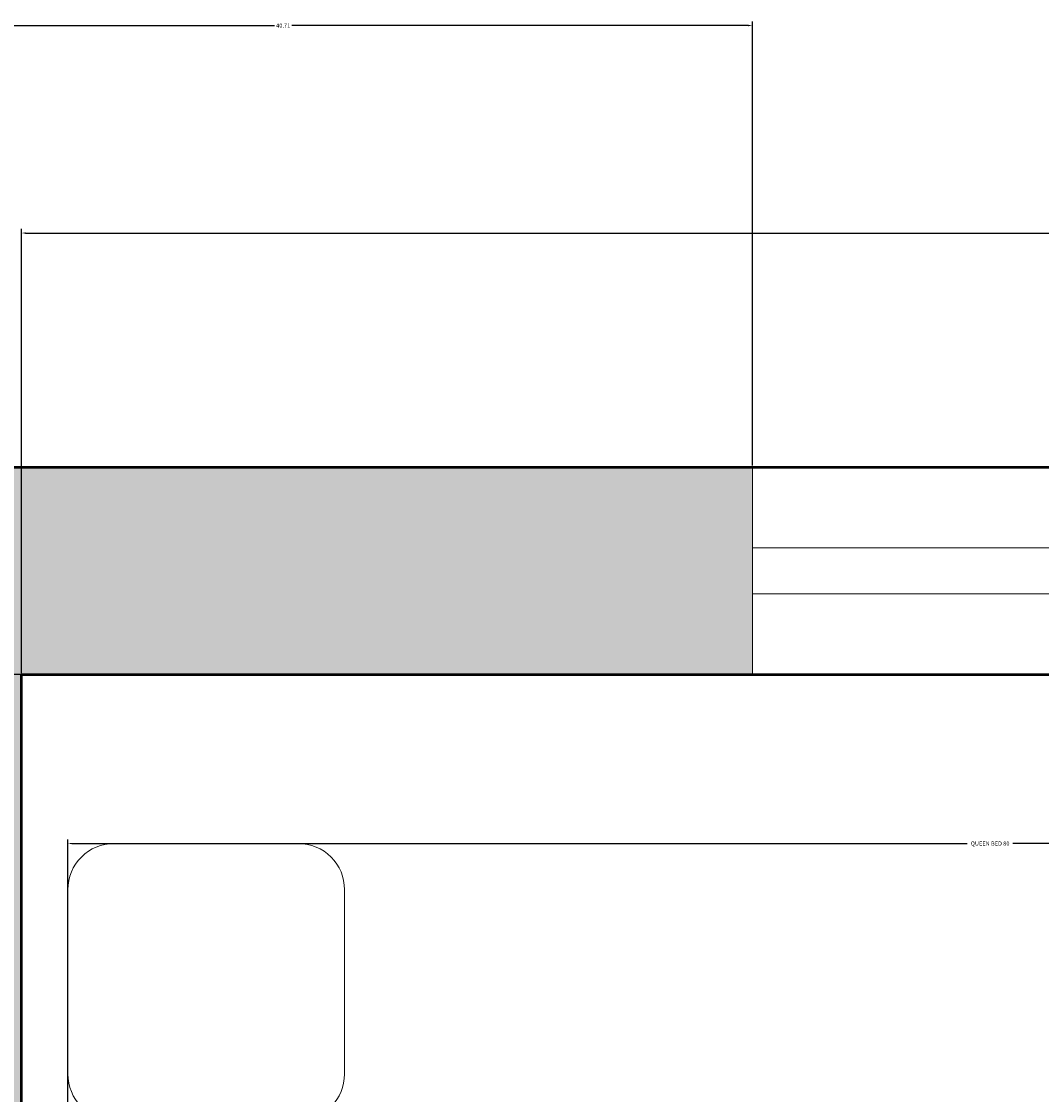
# Model space of a CAD drawing. Units: inches. Extents: x 2307 to 2544, y 2171 to 2540.
# Tile 24 of 52: x 2336 to 2380, y 2493 to 2540. Entities that reach past the tile are written whole.
import ezdxf

# ---------------------------------------------------------------- set-up
doc = ezdxf.new("R2010")
doc.units = ezdxf.units.IN
for name, color, linetype, lineweight in [('A-ANNO-DIMS', 2, 'Continuous', 18), ('A-FURN', 8, 'Continuous', 18), ('A-GLAZ', 4, 'Continuous', 18), ('A-WALL', 7, 'Continuous', 50)]:
    doc.layers.add(name, color=color, linetype=linetype, lineweight=lineweight)
doc.layers.add('A-WALL-PATT', color=18, linetype='Continuous', lineweight=13, true_color=0x000000)
doc.styles.get("Standard").update_dxf_attribs({"font": 'arial.ttf'})
doc.dimstyles.get("Standard").update_dxf_attribs({"dimtxt": 0.18, "dimasz": 0.18, "dimexe": 0.18, "dimexo": 0.0625, "dimgap": 0.09, "dimtad": 0, "dimtih": 1, "dimtoh": 1, "dimdec": 4, "dimzin": 0, "dimdsep": 46, "dimtxsty": 'Standard', "dimcen": 0.09, "dimadec": 0, "dimazin": 0, "dimtfac": 1, "dimtdec": 4, "dimtofl": 0, "dimtmove": 0, "dimatfit": 3, "dimfxl": 1, "dimtolj": 1, "dimtzin": 0, "dimarcsym": 0})

# ---------------------------------------------------------------- blocks, each defined once
blk = doc.blocks.new('WIN-48IN')
for p, q in [((0, 5.5), (48, 5.5)), ((0, 3.5), (48, 3.5))]:
    blk.add_line(p, q)
for points in [[(0, 0), (0, 9)], [(48, 9), (48, 0)]]:
    blk.add_lwpolyline(points)
blk = doc.blocks.new('*D26')
at = {"layer": 'A-ANNO-DIMS', "color": 0, "lineweight": -2, "transparency": 16777216}
for p, q in [((2337.708, 2492.237), (2337.708, 2504.354)), ((2417.708, 2492.237), (2417.708, 2504.354)), ((2337.888, 2504.174), (2376.714, 2504.174)), ((2417.528, 2504.174), (2378.702, 2504.174))]:
    blk.add_line(p, q, dxfattribs=at)
at = {"layer": 'A-ANNO-DIMS', "color": 0, "transparency": 16777216}
for points in [[(2337.888, 2504.204), (2337.888, 2504.144), (2337.708, 2504.174)], [(2417.528, 2504.204), (2417.528, 2504.144), (2417.708, 2504.174)]]:
    blk.add_solid(points, dxfattribs=at)
at = {"layer": 'Defpoints', "color": 0, "transparency": 16777216}
for p in [(2337.708, 2504.174), (2337.708, 2492.174), (2417.708, 2492.174)]:
    blk.add_point(p, dxfattribs=at)
at = {"layer": 'A-ANNO-DIMS', "color": 0, "transparency": 16777216, "insert": (2377.708, 2504.174), "char_height": 0.18, "attachment_point": 5}
blk.add_mtext('\\A1;QUEEN BED 80', dxfattribs=at)
blk = doc.blocks.new('*D42')
at = {"layer": 'A-ANNO-DIMS', "color": 0, "lineweight": -2, "transparency": 16777216}
for p, q in [((2326.696, 2520.572), (2326.696, 2539.84)), ((2326.876, 2539.66), (2346.669, 2539.66)), ((2367.223, 2539.66), (2347.429, 2539.66)), ((2367.403, 2520.572), (2367.403, 2539.84))]:
    blk.add_line(p, q, dxfattribs=at)
at = {"layer": 'A-ANNO-DIMS', "color": 0, "transparency": 16777216}
for points in [[(2326.876, 2539.69), (2326.876, 2539.63), (2326.696, 2539.66)], [(2367.223, 2539.69), (2367.223, 2539.63), (2367.403, 2539.66)]]:
    blk.add_solid(points, dxfattribs=at)
at = {"layer": 'Defpoints', "color": 0, "transparency": 16777216}
for p in [(2367.403, 2539.66), (2326.696, 2520.51), (2367.403, 2520.51)]:
    blk.add_point(p, dxfattribs=at)
at = {"layer": 'A-ANNO-DIMS', "color": 0, "transparency": 16777216, "insert": (2347.049, 2539.66), "char_height": 0.18, "attachment_point": 5}
blk.add_mtext('\\A1;40.71', dxfattribs=at)
blk = doc.blocks.new('*D45')
at = {"layer": 'A-ANNO-DIMS', "color": 0, "lineweight": -2, "transparency": 16777216}
for p, q in [((2335.696, 2511.572), (2335.696, 2530.84)), ((2451.696, 2511.572), (2451.696, 2530.84)), ((2335.876, 2530.66), (2393.416, 2530.66)), ((2451.516, 2530.66), (2393.976, 2530.66))]:
    blk.add_line(p, q, dxfattribs=at)
at = {"layer": 'A-ANNO-DIMS', "color": 0, "transparency": 16777216}
for points in [[(2335.876, 2530.69), (2335.876, 2530.63), (2335.696, 2530.66)], [(2451.516, 2530.69), (2451.516, 2530.63), (2451.696, 2530.66)]]:
    blk.add_solid(points, dxfattribs=at)
at = {"layer": 'Defpoints', "color": 0, "transparency": 16777216}
for p in [(2451.696, 2530.66), (2335.696, 2511.51), (2451.696, 2511.51)]:
    blk.add_point(p, dxfattribs=at)
at = {"layer": 'A-ANNO-DIMS', "color": 0, "transparency": 16777216, "insert": (2393.696, 2530.66), "char_height": 0.18, "attachment_point": 5}
blk.add_mtext('\\A1;116', dxfattribs=at)
blk = doc.blocks.new('*D48')
at = {"layer": 'A-ANNO-DIMS', "color": 0, "lineweight": -2, "transparency": 16777216}
for p, q in [((2455.633, 2511.51), (2307.366, 2511.51)), ((2307.546, 2511.33), (2307.546, 2475.69)), ((2307.546, 2439.69), (2307.546, 2475.329)), ((2455.633, 2439.51), (2307.366, 2439.51))]:
    blk.add_line(p, q, dxfattribs=at)
at = {"layer": 'A-ANNO-DIMS', "color": 0, "transparency": 16777216}
for points in [[(2307.516, 2511.33), (2307.576, 2511.33), (2307.546, 2511.51)], [(2307.516, 2439.69), (2307.576, 2439.69), (2307.546, 2439.51)]]:
    blk.add_solid(points, dxfattribs=at)
at = {"layer": 'Defpoints', "color": 0, "transparency": 16777216}
for p in [(2307.546, 2511.51), (2455.696, 2511.51), (2455.696, 2439.51)]:
    blk.add_point(p, dxfattribs=at)
at = {"layer": 'A-ANNO-DIMS', "color": 0, "transparency": 16777216, "insert": (2307.546, 2475.51), "char_height": 0.18, "attachment_point": 5}
blk.add_mtext('\\A1;72', dxfattribs=at)

msp = doc.modelspace()

# ---------------------------------------------------------------- hatches: boundary and pattern name
at = {"layer": 'A-WALL-PATT'}
h = msp.add_hatch(color=256, dxfattribs=at)
h.dxf.hatch_style = 1
h.paths.add_polyline_path([(2367.4028, 2520.5096), (2326.6958, 2520.5096), (2326.6958, 2355.3983), (2335.6958, 2355.3983), (2335.6958, 2387.5096), (2415.6958, 2387.5096), (2415.6958, 2391.5096), (2335.6958, 2391.5096), (2335.6958, 2409.5096), (2335.6958, 2511.5096), (2367.4028, 2511.5096)])

# ---------------------------------------------------------------- linework, layer by layer
at = {"layer": 'A-FURN'}
msp.add_lwpolyline([(2339.7083, 2492.1742), (2347.7083, 2492.1742, 0.4142136), (2349.7083, 2494.1742), (2349.7083, 2502.1742, 0.4142136), (2347.7083, 2504.1742), (2339.7083, 2504.1742, 0.4142136), (2337.7083, 2502.1742), (2337.7083, 2494.1742, 0.4142136)], format="xyb", close=True, dxfattribs=at)
at = {"layer": 'A-WALL'}
for p, q in [((2335.6958, 2511.5096), (2451.6958, 2511.5096)), ((2335.6958, 2391.5096), (2335.6958, 2511.5096))]:
    msp.add_line(p, q, dxfattribs=at)
msp.add_lwpolyline([(2433.7832, 2190.5096), (2326.6958, 2190.5096), (2326.6958, 2520.5096), (2524.6958, 2520.5096), (2524.6958, 2190.5096), (2469.785, 2190.5096)], dxfattribs=at)

# ---------------------------------------------------------------- block references
at = {"layer": 'A-GLAZ', "rotation": 180}
msp.add_blockref('WIN-48IN', (2415.4031, 2520.5091), dxfattribs=at)

# ---------------------------------------------------------------- dimensions: what is measured, and where the dimension line sits
at = {"layer": 'A-ANNO-DIMS'}
for base, p1, p2, override, picture, middle in [((2367.4028, 2539.6596), (2326.6958, 2520.5096), (2367.4028, 2520.5096), {"dimdec": 2, "dimlfac": 1, "dimrnd": 0, "dimzin": 0, "dimdsep": 46, "dimlunit": 2}, '*D42', (2347.0493, 2539.6596)), ((2451.6958, 2530.6596), (2335.6958, 2511.5096), (2451.6958, 2511.5096), {"dimdec": 0, "dimlfac": 1, "dimrnd": 0, "dimzin": 0, "dimdsep": 46, "dimlunit": 2}, '*D45', (2393.6958, 2530.6596))]:
    dim = msp.add_linear_dim(base=base, p1=p1, p2=p2, dimstyle='Standard', override=override, dxfattribs=at)
    dim.commit()
    dim.dimension.update_dxf_attribs({"geometry": picture, "text_midpoint": middle})
dim = msp.add_linear_dim(base=(2307.5458, 2511.5096), p1=(2455.6958, 2439.5096), p2=(2455.6958, 2511.5096), angle=90, dimstyle='Standard', override={"dimdec": 0, "dimlfac": 1, "dimrnd": 0, "dimzin": 0, "dimdsep": 46, "dimlunit": 2}, dxfattribs=at)
dim.commit()
dim.dimension.update_dxf_attribs({"geometry": '*D48', "text_midpoint": (2307.5458, 2475.5096)})
dim = msp.add_linear_dim(base=(2337.7083, 2504.1742), p1=(2417.7084, 2492.1742), p2=(2337.7083, 2492.1742), angle=180, text='QUEEN BED <>', dimstyle='Standard', override={"dimdec": 0, "dimlfac": 1, "dimrnd": 0, "dimzin": 0, "dimdsep": 46, "dimlunit": 2}, dxfattribs=at)
dim.commit()
dim.dimension.update_dxf_attribs({"geometry": '*D26', "text_midpoint": (2377.7083, 2504.1742)})

doc.saveas('drawing.dxf')
